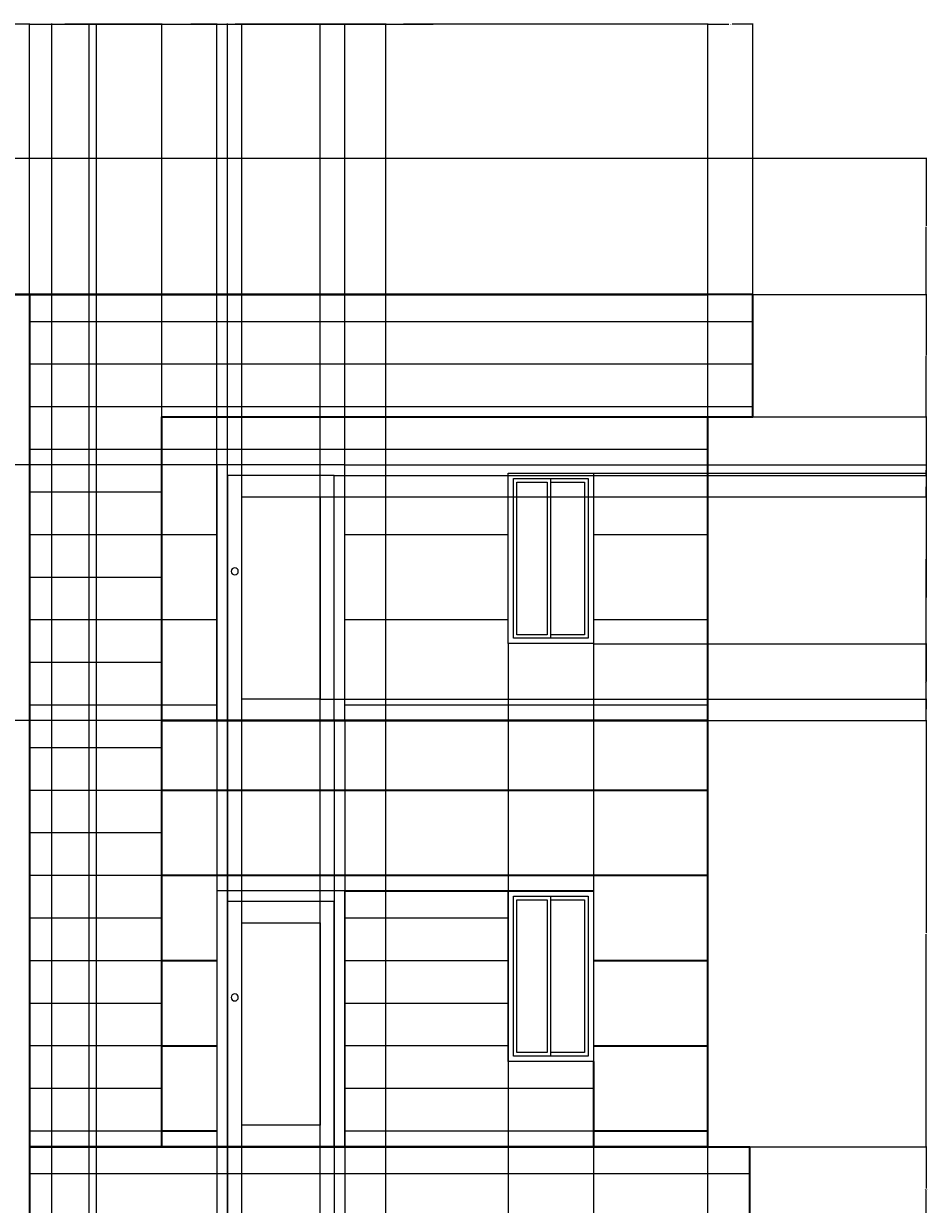
# Model space of a CAD drawing. Units: inches. Extents: x 10 to 404, y -77 to 696.
# Tile 5 of 5: x 149 to 404, y 363 to 696. Entities that reach past the tile are written whole.
import ezdxf

# ---------------------------------------------------------------- set-up
doc = ezdxf.new("R2010")
doc.units = ezdxf.units.IN
doc.header["$MEASUREMENT"] = 0
for name, color, linetype, lineweight in [('A-ANNO-DIMS', 2, 'Continuous', 18), ('A-DOOR', 4, 'Continuous', 25), ('A-ELEV', 7, 'Continuous', 35), ('A-ELEV-PATT', 8, 'Continuous', 13), ('A-GLAZ', 4, 'Continuous', 25)]:
    doc.layers.add(name, color=color, linetype=linetype, lineweight=lineweight)
doc.styles.get("Standard").update_dxf_attribs({"font": 'arial.ttf'})
doc.dimstyles.get("Standard").update_dxf_attribs({"dimtxt": 0.18, "dimasz": 0.18, "dimexe": 0.18, "dimexo": 0.0625, "dimgap": 0.09, "dimtad": 0, "dimtih": 1, "dimtoh": 1, "dimdec": 4, "dimzin": 0, "dimdsep": 46, "dimtxsty": 'Standard', "dimcen": 0.09, "dimadec": 0, "dimazin": 0, "dimtfac": 1, "dimtdec": 4, "dimtofl": 0, "dimtmove": 0, "dimatfit": 3, "dimfxl": 1, "dimtolj": 1, "dimtzin": 0, "dimarcsym": 0})

# ---------------------------------------------------------------- blocks, each defined once
blk = doc.blocks.new('*U5')
for p, q in [((1.5, 1.5), (1.5, 46.5)), ((1.5, 46.5), (12, 46.5)), ((12, 1.5), (12, 46.5)), ((12, 46.5), (22.5, 46.5)), ((22.5, 46.5), (22.5, 1.5)), ((12, 1.5), (1.5, 1.5)), ((22.5, 1.5), (12, 1.5))]:
    blk.add_line(p, q)
blk.add_lwpolyline([(0, 0), (0, 48), (24, 48), (24, 0)], close=True)
for points in [[(11, 45.5), (11, 2.5), (2.5, 2.5), (2.5, 45.5), (11, 45.5)], [(12, 45.5), (21.5, 45.5), (21.5, 2.5), (12, 2.5)]]:
    blk.add_lwpolyline(points)
blk = doc.blocks.new('*U4')
blk.add_lwpolyline([(3.12, 0.01), (0.12, 0.01), (0.12, 72.01), (36.12, 72.01), (36.12, 0.01), (33.12, 0.01)])
for points in [[(33.12, 68.99), (33.12, 0.01), (3.12, 0.01), (3.12, 68.99)], [(29.12, 6.01), (29.12, 62.99), (7.12, 62.99), (7.12, 6.01)]]:
    blk.add_lwpolyline(points, close=True)
blk.add_circle((31.12, 42.01), 1)
blk = doc.blocks.new('*D10')
at = {"layer": 'A-ANNO-DIMS', "color": 0, "lineweight": -2, "transparency": 16777216}
for p, q in [((65.94, 657.96), (9.76, 657.96)), ((9.94, 657.78), (9.94, 315.77)), ((9.94, -26.6), (9.94, 315.41)), ((176.46, -26.78), (9.76, -26.78))]:
    blk.add_line(p, q, dxfattribs=at)
at = {"layer": 'A-ANNO-DIMS', "color": 0, "transparency": 16777216}
for points in [[(9.91, 657.78), (9.97, 657.78), (9.94, 657.96)], [(9.91, -26.6), (9.97, -26.6), (9.94, -26.78)]]:
    blk.add_solid(points, dxfattribs=at)
at = {"layer": 'Defpoints', "color": 0, "transparency": 16777216}
for p in [(9.94, 657.96), (66.01, 657.96), (176.53, -26.78)]:
    blk.add_point(p, dxfattribs=at)
at = {"layer": 'A-ANNO-DIMS', "color": 0, "transparency": 16777216, "insert": (9.94, 315.59), "char_height": 0.18, "attachment_point": 5}
blk.add_mtext('\\A1;684.7', dxfattribs=at)
blk = doc.blocks.new('*D18')
at = {"layer": 'A-ANNO-DIMS', "color": 0, "lineweight": -2, "transparency": 16777216}
for p, q in [((78.1, 619.62), (78.1, 695.87)), ((78.28, 695.69), (114.12, 695.69)), ((150.75, 695.69), (114.91, 695.69)), ((150.93, 619.62), (150.93, 695.87))]:
    blk.add_line(p, q, dxfattribs=at)
at = {"layer": 'A-ANNO-DIMS', "color": 0, "transparency": 16777216}
for points in [[(78.28, 695.72), (78.28, 695.66), (78.1, 695.69)], [(150.75, 695.72), (150.75, 695.66), (150.93, 695.69)]]:
    blk.add_solid(points, dxfattribs=at)
at = {"layer": 'Defpoints', "color": 0, "transparency": 16777216}
for p in [(150.93, 695.69), (78.1, 619.55), (150.93, 619.55)]:
    blk.add_point(p, dxfattribs=at)
at = {"layer": 'A-ANNO-DIMS', "color": 0, "transparency": 16777216, "insert": (114.52, 695.69), "char_height": 0.18, "attachment_point": 5}
blk.add_mtext('\\A1;72.83', dxfattribs=at)
blk = doc.blocks.new('*D19')
at = {"layer": 'A-ANNO-DIMS', "color": 0, "lineweight": -2, "transparency": 16777216}
for p, q in [((150.93, 619.62), (150.93, 695.87)), ((151.11, 695.69), (169.13, 695.69)), ((187.94, 695.69), (169.92, 695.69)), ((188.12, 585.2), (188.12, 695.87))]:
    blk.add_line(p, q, dxfattribs=at)
at = {"layer": 'A-ANNO-DIMS', "color": 0, "transparency": 16777216}
for points in [[(151.11, 695.72), (151.11, 695.66), (150.93, 695.69)], [(187.94, 695.72), (187.94, 695.66), (188.12, 695.69)]]:
    blk.add_solid(points, dxfattribs=at)
at = {"layer": 'Defpoints', "color": 0, "transparency": 16777216}
for p in [(188.12, 695.69), (150.93, 619.55), (188.12, 585.13)]:
    blk.add_point(p, dxfattribs=at)
at = {"layer": 'A-ANNO-DIMS', "color": 0, "transparency": 16777216, "insert": (169.53, 695.69), "char_height": 0.18, "attachment_point": 5}
blk.add_mtext('\\A1;37.18', dxfattribs=at)
blk = doc.blocks.new('*D20')
at = {"layer": 'A-ANNO-DIMS', "color": 0, "lineweight": -2, "transparency": 16777216}
for p, q in [((188.12, 585.2), (188.12, 695.87)), ((188.3, 695.69), (264.54, 695.69)), ((341.69, 695.69), (265.45, 695.69)), ((341.87, 585.2), (341.87, 695.87))]:
    blk.add_line(p, q, dxfattribs=at)
at = {"layer": 'A-ANNO-DIMS', "color": 0, "transparency": 16777216}
for points in [[(188.3, 695.72), (188.3, 695.66), (188.12, 695.69)], [(341.69, 695.72), (341.69, 695.66), (341.87, 695.69)]]:
    blk.add_solid(points, dxfattribs=at)
at = {"layer": 'Defpoints', "color": 0, "transparency": 16777216}
for p in [(341.87, 695.69), (188.12, 585.13), (341.87, 585.13)]:
    blk.add_point(p, dxfattribs=at)
at = {"layer": 'A-ANNO-DIMS', "color": 0, "transparency": 16777216, "insert": (264.99, 695.69), "char_height": 0.18, "attachment_point": 5}
blk.add_mtext('\\A1;153.75', dxfattribs=at)
blk = doc.blocks.new('*D21')
at = {"layer": 'A-ANNO-DIMS', "color": 0, "lineweight": -2, "transparency": 16777216}
for p, q in [((341.87, 585.2), (341.87, 695.87)), ((342.05, 695.69), (347.76, 695.69)), ((354.38, 695.69), (348.67, 695.69)), ((354.56, 619.62), (354.56, 695.87))]:
    blk.add_line(p, q, dxfattribs=at)
at = {"layer": 'A-ANNO-DIMS', "color": 0, "transparency": 16777216}
for points in [[(342.05, 695.72), (342.05, 695.66), (341.87, 695.69)], [(354.38, 695.72), (354.38, 695.66), (354.56, 695.69)]]:
    blk.add_solid(points, dxfattribs=at)
at = {"layer": 'Defpoints', "color": 0, "transparency": 16777216}
for p in [(354.56, 695.69), (354.56, 619.55), (341.87, 585.13)]:
    blk.add_point(p, dxfattribs=at)
at = {"layer": 'A-ANNO-DIMS', "color": 0, "transparency": 16777216, "insert": (348.21, 695.69), "char_height": 0.18, "attachment_point": 5}
blk.add_mtext('\\A1;12.696', dxfattribs=at)
blk = doc.blocks.new('*D22')
at = {"layer": 'A-ANNO-DIMS', "color": 0, "lineweight": -2, "transparency": 16777216}
for p, q in [((188.12, 499.62), (188.12, 695.87)), ((188.3, 695.69), (195.51, 695.69)), ((203.49, 695.69), (196.28, 695.69)), ((203.67, 499.67), (203.67, 695.87))]:
    blk.add_line(p, q, dxfattribs=at)
at = {"layer": 'A-ANNO-DIMS', "color": 0, "transparency": 16777216}
for points in [[(188.3, 695.72), (188.3, 695.66), (188.12, 695.69)], [(203.49, 695.72), (203.49, 695.66), (203.67, 695.69)]]:
    blk.add_solid(points, dxfattribs=at)
at = {"layer": 'Defpoints', "color": 0, "transparency": 16777216}
for p in [(203.67, 695.69), (188.12, 499.55), (203.67, 499.6)]:
    blk.add_point(p, dxfattribs=at)
at = {"layer": 'A-ANNO-DIMS', "color": 0, "transparency": 16777216, "insert": (195.89, 695.69), "char_height": 0.18, "attachment_point": 5}
blk.add_mtext('\\A1;15.55', dxfattribs=at)
blk = doc.blocks.new('*D31')
at = {"layer": 'A-ANNO-DIMS', "color": 0, "lineweight": -2, "transparency": 16777216}
for p, q in [((353.65, 379.55), (403.47, 379.55)), ((403.29, 379.37), (403.29, 367.75)), ((403.29, 355.76), (403.29, 367.38)), ((353.65, 355.58), (403.47, 355.58))]:
    blk.add_line(p, q, dxfattribs=at)
at = {"layer": 'A-ANNO-DIMS', "color": 0, "transparency": 16777216}
for points in [[(403.26, 379.37), (403.32, 379.37), (403.29, 379.55)], [(403.26, 355.76), (403.32, 355.76), (403.29, 355.58)]]:
    blk.add_solid(points, dxfattribs=at)
at = {"layer": 'Defpoints', "color": 0, "transparency": 16777216}
for p in [(353.59, 379.55), (403.29, 379.55), (353.59, 355.58)]:
    blk.add_point(p, dxfattribs=at)
at = {"layer": 'A-ANNO-DIMS', "color": 0, "transparency": 16777216, "insert": (403.29, 367.57), "char_height": 0.18, "attachment_point": 5}
blk.add_mtext('\\A1;23.975', dxfattribs=at)
blk = doc.blocks.new('*D32')
at = {"layer": 'A-ANNO-DIMS', "color": 0, "lineweight": -2, "transparency": 16777216}
for p, q in [((341.93, 499.55), (403.47, 499.55)), ((403.29, 499.37), (403.29, 439.74)), ((403.29, 379.73), (403.29, 439.37)), ((341.93, 379.55), (403.47, 379.55))]:
    blk.add_line(p, q, dxfattribs=at)
at = {"layer": 'A-ANNO-DIMS', "color": 0, "transparency": 16777216}
for points in [[(403.26, 499.37), (403.32, 499.37), (403.29, 499.55)], [(403.26, 379.73), (403.32, 379.73), (403.29, 379.55)]]:
    blk.add_solid(points, dxfattribs=at)
at = {"layer": 'Defpoints', "color": 0, "transparency": 16777216}
for p in [(341.87, 499.55), (403.29, 499.55), (341.87, 379.55)]:
    blk.add_point(p, dxfattribs=at)
at = {"layer": 'A-ANNO-DIMS', "color": 0, "transparency": 16777216, "insert": (403.29, 439.55), "char_height": 0.18, "attachment_point": 5}
blk.add_mtext('\\A1;120', dxfattribs=at)
blk = doc.blocks.new('*D33')
at = {"layer": 'A-ANNO-DIMS', "color": 0, "lineweight": -2, "transparency": 16777216}
for p, q in [((354.63, 585.13), (403.47, 585.13)), ((403.29, 584.95), (403.29, 542.53)), ((403.29, 499.73), (403.29, 542.16)), ((341.93, 499.55), (403.47, 499.55))]:
    blk.add_line(p, q, dxfattribs=at)
at = {"layer": 'A-ANNO-DIMS', "color": 0, "transparency": 16777216}
for points in [[(403.26, 584.95), (403.32, 584.95), (403.29, 585.13)], [(403.26, 499.73), (403.32, 499.73), (403.29, 499.55)]]:
    blk.add_solid(points, dxfattribs=at)
at = {"layer": 'Defpoints', "color": 0, "transparency": 16777216}
for p in [(354.56, 585.13), (403.29, 585.13), (341.87, 499.55)]:
    blk.add_point(p, dxfattribs=at)
at = {"layer": 'A-ANNO-DIMS', "color": 0, "transparency": 16777216, "insert": (403.29, 542.34), "char_height": 0.18, "attachment_point": 5}
blk.add_mtext('\\A1;85.58', dxfattribs=at)
blk = doc.blocks.new('*D34')
at = {"layer": 'A-ANNO-DIMS', "color": 0, "lineweight": -2, "transparency": 16777216}
for p, q in [((354.63, 619.55), (403.47, 619.55)), ((403.29, 619.37), (403.29, 602.53)), ((403.29, 585.31), (403.29, 602.16)), ((354.63, 585.13), (403.47, 585.13))]:
    blk.add_line(p, q, dxfattribs=at)
at = {"layer": 'A-ANNO-DIMS', "color": 0, "transparency": 16777216}
for points in [[(403.26, 619.37), (403.32, 619.37), (403.29, 619.55)], [(403.26, 585.31), (403.32, 585.31), (403.29, 585.13)]]:
    blk.add_solid(points, dxfattribs=at)
at = {"layer": 'Defpoints', "color": 0, "transparency": 16777216}
for p in [(354.56, 619.55), (403.29, 619.55), (354.56, 585.13)]:
    blk.add_point(p, dxfattribs=at)
at = {"layer": 'A-ANNO-DIMS', "color": 0, "transparency": 16777216, "insert": (403.29, 602.34), "char_height": 0.18, "attachment_point": 5}
blk.add_mtext('\\A1;34.42', dxfattribs=at)
blk = doc.blocks.new('*D35')
at = {"layer": 'A-ANNO-DIMS', "color": 0, "lineweight": -2, "transparency": 16777216}
for p, q in [((66.07, 657.96), (403.47, 657.96)), ((403.29, 657.78), (403.29, 638.94)), ((403.29, 619.73), (403.29, 638.58)), ((354.63, 619.55), (403.47, 619.55))]:
    blk.add_line(p, q, dxfattribs=at)
at = {"layer": 'A-ANNO-DIMS', "color": 0, "transparency": 16777216}
for points in [[(403.26, 657.78), (403.32, 657.78), (403.29, 657.96)], [(403.26, 619.73), (403.32, 619.73), (403.29, 619.55)]]:
    blk.add_solid(points, dxfattribs=at)
at = {"layer": 'Defpoints', "color": 0, "transparency": 16777216}
for p in [(66.01, 657.96), (403.29, 657.96), (354.56, 619.55)]:
    blk.add_point(p, dxfattribs=at)
at = {"layer": 'A-ANNO-DIMS', "color": 0, "transparency": 16777216, "insert": (403.29, 638.76), "char_height": 0.18, "attachment_point": 5}
blk.add_mtext('\\A1;38.41', dxfattribs=at)
blk = doc.blocks.new('*D40')
at = {"layer": 'A-ANNO-DIMS', "color": 0, "lineweight": -2, "transparency": 16777216}
for p, q in [((150.93, 259.62), (150.93, 695.87)), ((151.11, 695.69), (159.89, 695.69)), ((169.58, 695.69), (160.8, 695.69)), ((169.76, 289.65), (169.76, 695.87))]:
    blk.add_line(p, q, dxfattribs=at)
at = {"layer": 'A-ANNO-DIMS', "color": 0, "transparency": 16777216}
for points in [[(151.11, 695.72), (151.11, 695.66), (150.93, 695.69)], [(169.58, 695.72), (169.58, 695.66), (169.76, 695.69)]]:
    blk.add_solid(points, dxfattribs=at)
at = {"layer": 'Defpoints', "color": 0, "transparency": 16777216}
for p in [(169.76, 695.69), (169.76, 289.59), (150.93, 259.55)]:
    blk.add_point(p, dxfattribs=at)
at = {"layer": 'A-ANNO-DIMS', "color": 0, "transparency": 16777216, "insert": (160.35, 695.69), "char_height": 0.18, "attachment_point": 5}
blk.add_mtext('\\A1;18.827', dxfattribs=at)
blk = doc.blocks.new('*D41')
at = {"layer": 'A-ANNO-DIMS', "color": 0, "lineweight": -2, "transparency": 16777216}
for p, q in [((169.76, 289.65), (169.76, 695.87)), ((169.94, 695.69), (255.45, 695.69)), ((341.69, 695.69), (256.18, 695.69)), ((341.87, 289.65), (341.87, 695.87))]:
    blk.add_line(p, q, dxfattribs=at)
at = {"layer": 'A-ANNO-DIMS', "color": 0, "transparency": 16777216}
for points in [[(169.94, 695.72), (169.94, 695.66), (169.76, 695.69)], [(341.69, 695.72), (341.69, 695.66), (341.87, 695.69)]]:
    blk.add_solid(points, dxfattribs=at)
at = {"layer": 'Defpoints', "color": 0, "transparency": 16777216}
for p in [(341.87, 695.69), (169.76, 289.59), (341.87, 289.59)]:
    blk.add_point(p, dxfattribs=at)
at = {"layer": 'A-ANNO-DIMS', "color": 0, "transparency": 16777216, "insert": (255.81, 695.69), "char_height": 0.18, "attachment_point": 5}
blk.add_mtext('\\A1;172.1', dxfattribs=at)
blk = doc.blocks.new('*D46')
at = {"layer": 'A-ANNO-DIMS', "color": 0, "lineweight": -2, "transparency": 16777216}
for p, q in [((309.68, 521.23), (403.47, 521.23)), ((403.29, 521.05), (403.29, 510.6)), ((403.29, 499.78), (403.29, 510.24)), ((239.73, 499.6), (403.47, 499.6))]:
    blk.add_line(p, q, dxfattribs=at)
at = {"layer": 'A-ANNO-DIMS', "color": 0, "transparency": 16777216}
for points in [[(403.26, 521.05), (403.32, 521.05), (403.29, 521.23)], [(403.26, 499.78), (403.32, 499.78), (403.29, 499.6)]]:
    blk.add_solid(points, dxfattribs=at)
at = {"layer": 'Defpoints', "color": 0, "transparency": 16777216}
for p in [(309.62, 521.23), (239.67, 499.6), (403.29, 499.6)]:
    blk.add_point(p, dxfattribs=at)
at = {"layer": 'A-ANNO-DIMS', "color": 0, "transparency": 16777216, "insert": (403.29, 510.42), "char_height": 0.18, "attachment_point": 5}
blk.add_mtext('\\A1;21.63', dxfattribs=at)
blk = doc.blocks.new('*D47')
at = {"layer": 'A-ANNO-DIMS', "color": 0, "lineweight": -2, "transparency": 16777216}
for p, q in [((309.68, 569.23), (403.47, 569.23)), ((403.29, 569.05), (403.29, 545.42)), ((403.29, 521.41), (403.29, 545.05)), ((309.68, 521.23), (403.47, 521.23))]:
    blk.add_line(p, q, dxfattribs=at)
at = {"layer": 'A-ANNO-DIMS', "color": 0, "transparency": 16777216}
for points in [[(403.26, 569.05), (403.32, 569.05), (403.29, 569.23)], [(403.26, 521.41), (403.32, 521.41), (403.29, 521.23)]]:
    blk.add_solid(points, dxfattribs=at)
at = {"layer": 'Defpoints', "color": 0, "transparency": 16777216}
for p in [(309.62, 569.23), (403.29, 569.23), (309.62, 521.23)]:
    blk.add_point(p, dxfattribs=at)
at = {"layer": 'A-ANNO-DIMS', "color": 0, "transparency": 16777216, "insert": (403.29, 545.23), "char_height": 0.18, "attachment_point": 5}
blk.add_mtext('\\A1;48', dxfattribs=at)
blk = doc.blocks.new('*D48')
at = {"layer": 'A-ANNO-DIMS', "color": 0, "lineweight": -2, "transparency": 16777216}
for p, q in [((285.62, 521.17), (285.62, -64.31)), ((239.67, 499.54), (239.67, -64.31)), ((239.85, -64.13), (262.25, -64.13)), ((285.44, -64.13), (263.04, -64.13))]:
    blk.add_line(p, q, dxfattribs=at)
at = {"layer": 'A-ANNO-DIMS', "color": 0, "transparency": 16777216}
for points in [[(239.85, -64.1), (239.85, -64.16), (239.67, -64.13)], [(285.44, -64.1), (285.44, -64.16), (285.62, -64.13)]]:
    blk.add_solid(points, dxfattribs=at)
at = {"layer": 'Defpoints', "color": 0, "transparency": 16777216}
for p in [(285.62, 521.23), (239.67, 499.6), (285.62, -64.13)]:
    blk.add_point(p, dxfattribs=at)
at = {"layer": 'A-ANNO-DIMS', "color": 0, "transparency": 16777216, "insert": (262.64, -64.13), "char_height": 0.18, "attachment_point": 5}
blk.add_mtext('\\A1;45.95', dxfattribs=at)
blk = doc.blocks.new('*D49')
at = {"layer": 'A-ANNO-DIMS', "color": 0, "lineweight": -2, "transparency": 16777216}
for p, q in [((285.62, 521.17), (285.62, -64.31)), ((309.62, 521.17), (309.62, -64.31)), ((285.8, -64.13), (297.4, -64.13)), ((309.44, -64.13), (297.84, -64.13))]:
    blk.add_line(p, q, dxfattribs=at)
at = {"layer": 'A-ANNO-DIMS', "color": 0, "transparency": 16777216}
for points in [[(285.8, -64.1), (285.8, -64.16), (285.62, -64.13)], [(309.44, -64.1), (309.44, -64.16), (309.62, -64.13)]]:
    blk.add_solid(points, dxfattribs=at)
at = {"layer": 'Defpoints', "color": 0, "transparency": 16777216}
for p in [(285.62, 521.23), (309.62, 521.23), (309.62, -64.13)]:
    blk.add_point(p, dxfattribs=at)
at = {"layer": 'A-ANNO-DIMS', "color": 0, "transparency": 16777216, "insert": (297.62, -64.13), "char_height": 0.18, "attachment_point": 5}
blk.add_mtext('\\A1;24', dxfattribs=at)
blk = doc.blocks.new('*D50')
at = {"layer": 'A-ANNO-DIMS', "color": 0, "lineweight": -2, "transparency": 16777216}
for p, q in [((157.2, 100.31), (157.2, 695.87)), ((157.38, 695.69), (161.98, 695.69)), ((167.49, 695.69), (162.89, 695.69)), ((167.67, 91.62), (167.67, 695.87))]:
    blk.add_line(p, q, dxfattribs=at)
at = {"layer": 'A-ANNO-DIMS', "color": 0, "transparency": 16777216}
for points in [[(157.38, 695.72), (157.38, 695.66), (157.2, 695.69)], [(167.49, 695.72), (167.49, 695.66), (167.67, 695.69)]]:
    blk.add_solid(points, dxfattribs=at)
at = {"layer": 'Defpoints', "color": 0, "transparency": 16777216}
for p in [(167.67, 695.69), (157.2, 100.24), (167.67, 91.55)]:
    blk.add_point(p, dxfattribs=at)
at = {"layer": 'A-ANNO-DIMS', "color": 0, "transparency": 16777216, "insert": (162.43, 695.69), "char_height": 0.18, "attachment_point": 5}
blk.add_mtext('\\A1;10.469', dxfattribs=at)
blk = doc.blocks.new('*D51')
at = {"layer": 'A-ANNO-DIMS', "color": 0, "lineweight": -2, "transparency": 16777216}
for p, q in [((167.67, 91.62), (167.67, 695.87)), ((167.85, 695.69), (209.06, 695.69)), ((251.06, 695.69), (209.85, 695.69)), ((251.24, 100.31), (251.24, 695.87))]:
    blk.add_line(p, q, dxfattribs=at)
at = {"layer": 'A-ANNO-DIMS', "color": 0, "transparency": 16777216}
for points in [[(167.85, 695.72), (167.85, 695.66), (167.67, 695.69)], [(251.06, 695.72), (251.06, 695.66), (251.24, 695.69)]]:
    blk.add_solid(points, dxfattribs=at)
at = {"layer": 'Defpoints', "color": 0, "transparency": 16777216}
for p in [(251.24, 695.69), (251.24, 100.24), (167.67, 91.55)]:
    blk.add_point(p, dxfattribs=at)
at = {"layer": 'A-ANNO-DIMS', "color": 0, "transparency": 16777216, "insert": (209.45, 695.69), "char_height": 0.18, "attachment_point": 5}
blk.add_mtext('\\A1;83.57', dxfattribs=at)
blk = doc.blocks.new('*D61')
at = {"layer": 'A-ANNO-DIMS', "color": 0, "lineweight": -2, "transparency": 16777216}
for p, q in [((206.67, 19.62), (206.67, 695.87)), ((206.85, 695.69), (208.51, 695.69)), ((210.49, 695.69), (208.82, 695.69)), ((210.67, 25.62), (210.67, 695.87))]:
    blk.add_line(p, q, dxfattribs=at)
at = {"layer": 'A-ANNO-DIMS', "color": 0, "transparency": 16777216}
for points in [[(206.85, 695.72), (206.85, 695.66), (206.67, 695.69)], [(210.49, 695.72), (210.49, 695.66), (210.67, 695.69)]]:
    blk.add_solid(points, dxfattribs=at)
at = {"layer": 'Defpoints', "color": 0, "transparency": 16777216}
for p in [(210.67, 695.69), (210.67, 25.55), (206.67, 19.55)]:
    blk.add_point(p, dxfattribs=at)
at = {"layer": 'A-ANNO-DIMS', "color": 0, "transparency": 16777216, "insert": (208.67, 695.69), "char_height": 0.18, "attachment_point": 5}
blk.add_mtext('\\A1;4', dxfattribs=at)
blk = doc.blocks.new('*D62')
at = {"layer": 'A-ANNO-DIMS', "color": 0, "lineweight": -2, "transparency": 16777216}
for p, q in [((210.67, 25.62), (210.67, 695.87)), ((210.85, 695.69), (221.45, 695.69)), ((232.49, 695.69), (221.89, 695.69)), ((232.67, 25.62), (232.67, 695.87))]:
    blk.add_line(p, q, dxfattribs=at)
at = {"layer": 'A-ANNO-DIMS', "color": 0, "transparency": 16777216}
for points in [[(210.85, 695.72), (210.85, 695.66), (210.67, 695.69)], [(232.49, 695.72), (232.49, 695.66), (232.67, 695.69)]]:
    blk.add_solid(points, dxfattribs=at)
at = {"layer": 'Defpoints', "color": 0, "transparency": 16777216}
for p in [(232.67, 695.69), (210.67, 25.55), (232.67, 25.55)]:
    blk.add_point(p, dxfattribs=at)
at = {"layer": 'A-ANNO-DIMS', "color": 0, "transparency": 16777216, "insert": (221.67, 695.69), "char_height": 0.18, "attachment_point": 5}
blk.add_mtext('\\A1;22', dxfattribs=at)
blk = doc.blocks.new('*D65')
at = {"layer": 'A-ANNO-DIMS', "color": 0, "lineweight": -2, "transparency": 16777216}
for p, q in [((203.67, 571.67), (203.67, 695.87)), ((203.85, 695.69), (221.45, 695.69)), ((239.49, 695.69), (221.89, 695.69)), ((239.67, 571.67), (239.67, 695.87))]:
    blk.add_line(p, q, dxfattribs=at)
at = {"layer": 'A-ANNO-DIMS', "color": 0, "transparency": 16777216}
for points in [[(203.85, 695.72), (203.85, 695.66), (203.67, 695.69)], [(239.49, 695.72), (239.49, 695.66), (239.67, 695.69)]]:
    blk.add_solid(points, dxfattribs=at)
at = {"layer": 'Defpoints', "color": 0, "transparency": 16777216}
for p in [(239.67, 695.69), (203.67, 571.6), (239.67, 571.6)]:
    blk.add_point(p, dxfattribs=at)
at = {"layer": 'A-ANNO-DIMS', "color": 0, "transparency": 16777216, "insert": (221.67, 695.69), "char_height": 0.18, "attachment_point": 5}
blk.add_mtext('\\A1;36', dxfattribs=at)
blk = doc.blocks.new('*D66')
at = {"layer": 'A-ANNO-DIMS', "color": 0, "lineweight": -2, "transparency": 16777216}
for p, q in [((203.67, 499.54), (203.67, -64.31)), ((206.67, 499.54), (206.67, -64.31)), ((203.85, -64.13), (205.02, -64.13)), ((206.49, -64.13), (205.32, -64.13))]:
    blk.add_line(p, q, dxfattribs=at)
at = {"layer": 'A-ANNO-DIMS', "color": 0, "transparency": 16777216}
for points in [[(203.85, -64.1), (203.85, -64.16), (203.67, -64.13)], [(206.49, -64.1), (206.49, -64.16), (206.67, -64.13)]]:
    blk.add_solid(points, dxfattribs=at)
at = {"layer": 'Defpoints', "color": 0, "transparency": 16777216}
for p in [(203.67, 499.6), (206.67, 499.6), (206.67, -64.13)]:
    blk.add_point(p, dxfattribs=at)
at = {"layer": 'A-ANNO-DIMS', "color": 0, "transparency": 16777216, "insert": (205.17, -64.13), "char_height": 0.18, "attachment_point": 5}
blk.add_mtext('\\A1;3', dxfattribs=at)
blk = doc.blocks.new('*D67')
at = {"layer": 'A-ANNO-DIMS', "color": 0, "lineweight": -2, "transparency": 16777216}
for p, q in [((206.67, 499.54), (206.67, -64.31)), ((236.67, 499.54), (236.67, -64.31)), ((206.85, -64.13), (221.45, -64.13)), ((236.49, -64.13), (221.89, -64.13))]:
    blk.add_line(p, q, dxfattribs=at)
at = {"layer": 'A-ANNO-DIMS', "color": 0, "transparency": 16777216}
for points in [[(206.85, -64.1), (206.85, -64.16), (206.67, -64.13)], [(236.49, -64.1), (236.49, -64.16), (236.67, -64.13)]]:
    blk.add_solid(points, dxfattribs=at)
at = {"layer": 'Defpoints', "color": 0, "transparency": 16777216}
for p in [(206.67, 499.6), (236.67, 499.6), (236.67, -64.13)]:
    blk.add_point(p, dxfattribs=at)
at = {"layer": 'A-ANNO-DIMS', "color": 0, "transparency": 16777216, "insert": (221.67, -64.13), "char_height": 0.18, "attachment_point": 5}
blk.add_mtext('\\A1;30', dxfattribs=at)
blk = doc.blocks.new('*D68')
at = {"layer": 'A-ANNO-DIMS', "color": 0, "lineweight": -2, "transparency": 16777216}
for p, q in [((236.67, 499.54), (236.67, -64.31)), ((239.67, 499.54), (239.67, -64.31)), ((236.85, -64.13), (238.02, -64.13)), ((239.49, -64.13), (238.32, -64.13))]:
    blk.add_line(p, q, dxfattribs=at)
at = {"layer": 'A-ANNO-DIMS', "color": 0, "transparency": 16777216}
for points in [[(236.85, -64.1), (236.85, -64.16), (236.67, -64.13)], [(239.49, -64.1), (239.49, -64.16), (239.67, -64.13)]]:
    blk.add_solid(points, dxfattribs=at)
at = {"layer": 'Defpoints', "color": 0, "transparency": 16777216}
for p in [(236.67, 499.6), (239.67, 499.6), (239.67, -64.13)]:
    blk.add_point(p, dxfattribs=at)
at = {"layer": 'A-ANNO-DIMS', "color": 0, "transparency": 16777216, "insert": (238.17, -64.13), "char_height": 0.18, "attachment_point": 5}
blk.add_mtext('\\A1;3', dxfattribs=at)
blk = doc.blocks.new('*D69')
at = {"layer": 'A-ANNO-DIMS', "color": 0, "lineweight": -2, "transparency": 16777216}
for p, q in [((206.67, 499.67), (206.67, 695.87)), ((206.85, 695.69), (208.51, 695.69)), ((210.49, 695.69), (208.82, 695.69)), ((210.67, 505.67), (210.67, 695.87))]:
    blk.add_line(p, q, dxfattribs=at)
at = {"layer": 'A-ANNO-DIMS', "color": 0, "transparency": 16777216}
for points in [[(206.85, 695.72), (206.85, 695.66), (206.67, 695.69)], [(210.49, 695.72), (210.49, 695.66), (210.67, 695.69)]]:
    blk.add_solid(points, dxfattribs=at)
at = {"layer": 'Defpoints', "color": 0, "transparency": 16777216}
for p in [(210.67, 695.69), (210.67, 505.6), (206.67, 499.6)]:
    blk.add_point(p, dxfattribs=at)
at = {"layer": 'A-ANNO-DIMS', "color": 0, "transparency": 16777216, "insert": (208.67, 695.69), "char_height": 0.18, "attachment_point": 5}
blk.add_mtext('\\A1;4', dxfattribs=at)
blk = doc.blocks.new('*D70')
at = {"layer": 'A-ANNO-DIMS', "color": 0, "lineweight": -2, "transparency": 16777216}
for p, q in [((210.67, 505.67), (210.67, 695.87)), ((210.85, 695.69), (221.45, 695.69)), ((232.49, 695.69), (221.89, 695.69)), ((232.67, 505.67), (232.67, 695.87))]:
    blk.add_line(p, q, dxfattribs=at)
at = {"layer": 'A-ANNO-DIMS', "color": 0, "transparency": 16777216}
for points in [[(210.85, 695.72), (210.85, 695.66), (210.67, 695.69)], [(232.49, 695.72), (232.49, 695.66), (232.67, 695.69)]]:
    blk.add_solid(points, dxfattribs=at)
at = {"layer": 'Defpoints', "color": 0, "transparency": 16777216}
for p in [(232.67, 695.69), (210.67, 505.6), (232.67, 505.6)]:
    blk.add_point(p, dxfattribs=at)
at = {"layer": 'A-ANNO-DIMS', "color": 0, "transparency": 16777216, "insert": (221.67, 695.69), "char_height": 0.18, "attachment_point": 5}
blk.add_mtext('\\A1;22', dxfattribs=at)
blk = doc.blocks.new('*D71')
at = {"layer": 'A-ANNO-DIMS', "color": 0, "lineweight": -2, "transparency": 16777216}
for p, q in [((203.6, 571.6), (9.76, 571.6)), ((9.94, 571.42), (9.94, 535.78)), ((9.94, 499.78), (9.94, 535.42)), ((203.6, 499.6), (9.76, 499.6))]:
    blk.add_line(p, q, dxfattribs=at)
at = {"layer": 'A-ANNO-DIMS', "color": 0, "transparency": 16777216}
for points in [[(9.91, 571.42), (9.97, 571.42), (9.94, 571.6)], [(9.91, 499.78), (9.97, 499.78), (9.94, 499.6)]]:
    blk.add_solid(points, dxfattribs=at)
at = {"layer": 'Defpoints', "color": 0, "transparency": 16777216}
for p in [(9.94, 571.6), (203.67, 571.6), (203.67, 499.6)]:
    blk.add_point(p, dxfattribs=at)
at = {"layer": 'A-ANNO-DIMS', "color": 0, "transparency": 16777216, "insert": (9.94, 535.6), "char_height": 0.18, "attachment_point": 5}
blk.add_mtext('\\A1;72', dxfattribs=at)
blk = doc.blocks.new('*D72')
at = {"layer": 'A-ANNO-DIMS', "color": 0, "lineweight": -2, "transparency": 16777216}
for p, q in [((232.73, 505.6), (403.47, 505.6)), ((403.29, 505.42), (403.29, 502.79)), ((403.29, 499.78), (403.29, 502.42)), ((236.73, 499.6), (403.47, 499.6))]:
    blk.add_line(p, q, dxfattribs=at)
at = {"layer": 'A-ANNO-DIMS', "color": 0, "transparency": 16777216}
for points in [[(403.26, 505.42), (403.32, 505.42), (403.29, 505.6)], [(403.26, 499.78), (403.32, 499.78), (403.29, 499.6)]]:
    blk.add_solid(points, dxfattribs=at)
at = {"layer": 'Defpoints', "color": 0, "transparency": 16777216}
for p in [(232.67, 505.6), (403.29, 505.6), (236.67, 499.6)]:
    blk.add_point(p, dxfattribs=at)
at = {"layer": 'A-ANNO-DIMS', "color": 0, "transparency": 16777216, "insert": (403.29, 502.6), "char_height": 0.18, "attachment_point": 5}
blk.add_mtext('\\A1;6', dxfattribs=at)
blk = doc.blocks.new('*D73')
at = {"layer": 'A-ANNO-DIMS', "color": 0, "lineweight": -2, "transparency": 16777216}
for p, q in [((232.73, 562.58), (403.47, 562.58)), ((403.29, 562.4), (403.29, 534.27)), ((403.29, 505.78), (403.29, 533.91)), ((232.73, 505.6), (403.47, 505.6))]:
    blk.add_line(p, q, dxfattribs=at)
at = {"layer": 'A-ANNO-DIMS', "color": 0, "transparency": 16777216}
for points in [[(403.26, 562.4), (403.32, 562.4), (403.29, 562.58)], [(403.26, 505.78), (403.32, 505.78), (403.29, 505.6)]]:
    blk.add_solid(points, dxfattribs=at)
at = {"layer": 'Defpoints', "color": 0, "transparency": 16777216}
for p in [(232.67, 562.58), (403.29, 562.58), (232.67, 505.6)]:
    blk.add_point(p, dxfattribs=at)
at = {"layer": 'A-ANNO-DIMS', "color": 0, "transparency": 16777216, "insert": (403.29, 534.09), "char_height": 0.18, "attachment_point": 5}
blk.add_mtext('\\A1;56.98', dxfattribs=at)
blk = doc.blocks.new('*D74')
at = {"layer": 'A-ANNO-DIMS', "color": 0, "lineweight": -2, "transparency": 16777216}
for p, q in [((236.73, 568.58), (403.47, 568.58)), ((403.29, 568.4), (403.29, 565.76)), ((403.29, 562.76), (403.29, 565.4)), ((232.73, 562.58), (403.47, 562.58))]:
    blk.add_line(p, q, dxfattribs=at)
at = {"layer": 'A-ANNO-DIMS', "color": 0, "transparency": 16777216}
for points in [[(403.26, 568.4), (403.32, 568.4), (403.29, 568.58)], [(403.26, 562.76), (403.32, 562.76), (403.29, 562.58)]]:
    blk.add_solid(points, dxfattribs=at)
at = {"layer": 'Defpoints', "color": 0, "transparency": 16777216}
for p in [(236.67, 568.58), (403.29, 568.58), (232.67, 562.58)]:
    blk.add_point(p, dxfattribs=at)
at = {"layer": 'A-ANNO-DIMS', "color": 0, "transparency": 16777216, "insert": (403.29, 565.58), "char_height": 0.18, "attachment_point": 5}
blk.add_mtext('\\A1;6', dxfattribs=at)
blk = doc.blocks.new('*D75')
at = {"layer": 'A-ANNO-DIMS', "color": 0, "lineweight": -2, "transparency": 16777216}
for p, q in [((239.73, 571.6), (403.47, 571.6)), ((403.29, 571.42), (403.29, 570.28)), ((403.29, 568.76), (403.29, 569.91)), ((236.73, 568.58), (403.47, 568.58))]:
    blk.add_line(p, q, dxfattribs=at)
at = {"layer": 'A-ANNO-DIMS', "color": 0, "transparency": 16777216}
for points in [[(403.26, 571.42), (403.32, 571.42), (403.29, 571.6)], [(403.26, 568.76), (403.32, 568.76), (403.29, 568.58)]]:
    blk.add_solid(points, dxfattribs=at)
at = {"layer": 'Defpoints', "color": 0, "transparency": 16777216}
for p in [(239.67, 571.6), (403.29, 571.6), (236.67, 568.58)]:
    blk.add_point(p, dxfattribs=at)
at = {"layer": 'A-ANNO-DIMS', "color": 0, "transparency": 16777216, "insert": (403.29, 570.09), "char_height": 0.18, "attachment_point": 5}
blk.add_mtext('\\A1;3.023', dxfattribs=at)

msp = doc.modelspace()

# ---------------------------------------------------------------- hatches: boundary and pattern name
at = {"layer": 'A-ELEV-PATT'}
h = msp.add_hatch(dxfattribs=at)
h.set_pattern_fill('_USER', color=256, scale=12, pattern_type=0)
h.set_pattern_definition([(0, (0, 0), (0, 12), [])])
h.paths.add_polyline_path([(188.1159, 499.5535), (150.9344, 499.5535), (150.9344, 379.5535), (188.1159, 379.5535)])
h.paths.add_polyline_path([(188.1159, 585.1332), (354.5631, 585.1332), (354.5631, 619.5535), (341.8668, 619.5535), (150.9344, 619.5535), (150.9344, 499.5535), (188.1159, 499.5535)])
h.paths.add_polyline_path([(353.5898, 379.5535), (341.8668, 379.5535), (150.9344, 379.5535), (150.9344, 259.5535), (341.8668, 259.5535), (353.8668, 259.5535), (353.8668, 273.1993), (341.8668, 273.1993), (169.7618, 273.1993), (169.7618, 355.5535), (341.8668, 355.5535), (341.8668, 355.5783), (353.5898, 355.5783)])
h.paths.add_polyline_path([(285.6197, 451.5918), (239.6671, 451.5918), (239.6671, 379.5535), (309.6197, 379.5535), (309.6197, 403.5918), (285.6197, 403.5918)])
h.paths.add_polyline_path([(199.3943, 256.7444), (154.0619, 256.7444), (154.0619, 142.2479), (199.3943, 142.2479)])
h = msp.add_hatch(dxfattribs=at)
h.set_pattern_fill('_USER', color=256, scale=24, pattern_type=0)
h.set_pattern_definition([(0, (0, 0), (0, 24), [])])
h.paths.add_polyline_path([(341.8668, 139.5535), (150.9344, 139.5535), (150.9344, 19.5535), (167.6671, 19.5535), (167.6671, 91.5535), (157.1984, 91.5535), (157.1984, 100.244), (251.2392, 100.244), (251.2392, 91.5535), (239.6671, 91.5535), (239.6671, 19.5535), (341.8668, 19.5535)])
h.paths.add_polyline_path([(285.6197, 89.2337), (309.6197, 89.2337), (309.6197, 41.2337), (285.6197, 41.2337)], flags=16)
h.paths.add_polyline_path([(287.1197, 87.7337), (297.6197, 87.7337), (308.1197, 87.7337), (308.1197, 42.7337), (297.6197, 42.7337), (287.1197, 42.7337)], flags=0)
h.paths.add_polyline_path([(288.1197, 86.7337), (296.6197, 86.7337), (296.6197, 43.7337), (288.1197, 43.7337)], flags=0)
h.paths.add_polyline_path([(297.6197, 86.7337), (307.1197, 86.7337), (307.1197, 43.7337), (297.6197, 43.7337)], flags=0)
h.paths.add_polyline_path([(341.8668, 585.1332), (188.1159, 585.1332), (188.1159, 499.5535), (203.6671, 499.5535), (203.6671, 571.6046), (239.6671, 571.6046), (239.6671, 499.5535), (341.8668, 499.5535)])
h.paths.add_polyline_path([(285.6197, 521.2337), (285.6197, 569.2337), (309.6197, 569.2337), (309.6197, 521.2337)], flags=16)
h.paths.add_polyline_path([(287.1197, 522.7337), (287.1197, 567.7337), (297.6197, 567.7337), (308.1197, 567.7337), (308.1197, 522.7337), (297.6197, 522.7337)], flags=0)
h.paths.add_polyline_path([(288.1197, 523.7337), (288.1197, 566.7337), (296.6197, 566.7337), (296.6197, 523.7337)], flags=0)
h.paths.add_polyline_path([(297.6197, 566.7337), (307.1197, 566.7337), (307.1197, 523.7337), (297.6197, 523.7337)], flags=0)

# ---------------------------------------------------------------- linework, layer by layer
at = {"layer": 'A-ELEV'}
for p, q in [((341.8668, 619.5535), (78.1013, 619.5535)), ((78.1013, 619.5535), (341.8668, 619.5535)), ((150.9344, 19.5535), (150.9344, 619.5535)), ((354.5631, 619.5535), (341.8668, 619.5535)), ((354.5631, 585.1332), (354.5631, 619.5535)), ((188.1159, 379.5535), (188.1159, 585.1332)), ((188.1159, 585.1332), (354.5631, 585.1332)), ((341.8668, 499.5535), (341.8668, 585.1332)), ((341.8668, 499.5535), (188.1159, 499.5535)), ((188.1159, 499.5535), (341.8668, 499.5535)), ((341.8668, 379.5535), (341.8668, 499.5535)), ((188.1159, 480), (341.8668, 480)), ((188.1159, 456), (341.8668, 456)), ((239.6671, 451.5918), (309.6197, 451.5918)), ((188.1159, 432), (203.6671, 432)), ((309.6197, 432), (341.8668, 432)), ((188.1159, 408), (203.6671, 408)), ((309.6197, 408), (341.8668, 408)), ((309.6197, 403.5918), (309.6197, 379.5535)), ((188.1159, 384), (203.6671, 384)), ((309.6197, 384), (341.8668, 384)), ((341.8668, 379.5535), (150.9344, 379.5535)), ((150.9344, 379.5535), (341.8668, 379.5535))]:
    msp.add_line(p, q, dxfattribs=at)
msp.add_lwpolyline([(341.8668, 379.5535), (353.5898, 379.5535), (353.5898, 355.5783), (341.8668, 355.5783)], dxfattribs=at)

# ---------------------------------------------------------------- block references
at = {"layer": 'A-DOOR', "xscale": -1}
for p in [(239.7909, 499.5918), (239.7909, 379.5791)]:
    msp.add_blockref('*U4', p, dxfattribs=at)
at = {"layer": 'A-GLAZ'}
for p in [(285.6197, 521.2337), (285.6197, 403.5918)]:
    msp.add_blockref('*U5', p, dxfattribs=at)

# ---------------------------------------------------------------- dimensions: what is measured, and where the dimension line sits
at = {"layer": 'A-ANNO-DIMS'}
for base, p1, p2, override, picture, middle in [((150.9344, 695.6911), (78.1013, 619.5535), (150.9344, 619.5535), {"dimdec": 2, "dimlfac": 1, "dimrnd": 0, "dimzin": 0, "dimdsep": 46, "dimlunit": 2}, '*D18', (114.5179, 695.6911)), ((188.1159, 695.6911), (150.9344, 619.5535), (188.1159, 585.1332), {"dimdec": 2, "dimlfac": 1, "dimrnd": 0, "dimzin": 0, "dimdsep": 46, "dimlunit": 2}, '*D19', (169.5251, 695.6911)), ((169.7618, 695.6911), (150.9344, 259.5535), (169.7618, 289.5881), {"dimdec": 3, "dimlfac": 1, "dimrnd": 0, "dimzin": 0, "dimdsep": 46, "dimlunit": 2}, '*D40', (160.3481, 695.6911)), ((167.6671, 695.6911), (157.1984, 100.244), (167.6671, 91.5535), {"dimdec": 3, "dimlfac": 1, "dimrnd": 0, "dimzin": 0, "dimdsep": 46, "dimlunit": 2}, '*D50', (162.4328, 695.6911)), ((251.2392, 695.6911), (167.6671, 91.5535), (251.2392, 100.244), {"dimdec": 2, "dimlfac": 1, "dimrnd": 0, "dimzin": 0, "dimdsep": 46, "dimlunit": 2}, '*D51', (209.4531, 695.6911)), ((341.8668, 695.6911), (169.7618, 289.5881), (341.8668, 289.5881), {"dimdec": 1, "dimlfac": 1, "dimrnd": 0, "dimzin": 0, "dimdsep": 46, "dimlunit": 2}, '*D41', (255.8143, 695.6911)), ((341.8668, 695.6911), (188.1159, 585.1332), (341.8668, 585.1332), {"dimdec": 2, "dimlfac": 1, "dimrnd": 0, "dimzin": 0, "dimdsep": 46, "dimlunit": 2}, '*D20', (264.9913, 695.6911)), ((203.6671, 695.6911), (188.1159, 499.5535), (203.6671, 499.6046), {"dimdec": 2, "dimlfac": 1, "dimrnd": 0, "dimzin": 0, "dimdsep": 46, "dimlunit": 2}, '*D22', (195.8915, 695.6911)), ((239.6671, 695.6911), (203.6671, 571.6046), (239.6671, 571.6046), {"dimdec": 0, "dimlfac": 1, "dimrnd": 0, "dimzin": 0, "dimdsep": 46, "dimlunit": 2}, '*D65', (221.6671, 695.6911)), ((210.6671, 695.6911), (206.6671, 19.5535), (210.6671, 25.5535), {"dimdec": 0, "dimlfac": 1, "dimrnd": 0, "dimzin": 0, "dimdsep": 46, "dimlunit": 2}, '*D61', (208.6671, 695.6911)), ((210.6671, 695.6911), (206.6671, 499.6046), (210.6671, 505.6046), {"dimdec": 0, "dimlfac": 1, "dimrnd": 0, "dimzin": 0, "dimdsep": 46, "dimlunit": 2}, '*D69', (208.6671, 695.6911)), ((232.6671, 695.6911), (210.6671, 25.5535), (232.6671, 25.5535), {"dimdec": 0, "dimlfac": 1, "dimrnd": 0, "dimzin": 0, "dimdsep": 46, "dimlunit": 2}, '*D62', (221.6671, 695.6911)), ((232.6671, 695.6911), (210.6671, 505.6046), (232.6671, 505.6046), {"dimdec": 0, "dimlfac": 1, "dimrnd": 0, "dimzin": 0, "dimdsep": 46, "dimlunit": 2}, '*D70', (221.6671, 695.6911)), ((354.5631, 695.6911), (341.8668, 585.1332), (354.5631, 619.5535), {"dimdec": 3, "dimlfac": 1, "dimrnd": 0, "dimzin": 0, "dimdsep": 46, "dimlunit": 2}, '*D21', (348.2149, 695.6911)), ((285.6197, -64.1316), (239.6671, 499.6046), (285.6197, 521.2337), {"dimdec": 2, "dimlfac": 1, "dimrnd": 0, "dimzin": 0, "dimdsep": 46, "dimlunit": 2}, '*D48', (262.6434, -64.1316)), ((309.6197, -64.1316), (285.6197, 521.2337), (309.6197, 521.2337), {"dimdec": 0, "dimlfac": 1, "dimrnd": 0, "dimzin": 0, "dimdsep": 46, "dimlunit": 2}, '*D49', (297.6197, -64.1316)), ((206.6671, -64.1316), (203.6671, 499.6046), (206.6671, 499.6046), {"dimdec": 0, "dimlfac": 1, "dimrnd": 0, "dimzin": 0, "dimdsep": 46, "dimlunit": 2}, '*D66', (205.1671, -64.1316)), ((236.6671, -64.1316), (206.6671, 499.6046), (236.6671, 499.6046), {"dimdec": 0, "dimlfac": 1, "dimrnd": 0, "dimzin": 0, "dimdsep": 46, "dimlunit": 2}, '*D67', (221.6671, -64.1316)), ((239.6671, -64.1316), (236.6671, 499.6046), (239.6671, 499.6046), {"dimdec": 0, "dimlfac": 1, "dimrnd": 0, "dimzin": 0, "dimdsep": 46, "dimlunit": 2}, '*D68', (238.1671, -64.1316))]:
    dim = msp.add_linear_dim(base=base, p1=p1, p2=p2, dimstyle='Standard', override=override, dxfattribs=at)
    dim.commit()
    dim.dimension.update_dxf_attribs({"geometry": picture, "text_midpoint": middle})
for base, p1, p2, override, picture, middle in [((9.9405, 657.9612), (176.5266, -26.7816), (66.0062, 657.9612), {"dimdec": 1, "dimlfac": 1, "dimrnd": 0, "dimzin": 0, "dimdsep": 46, "dimlunit": 2}, '*D10', (9.9405, 315.5898)), ((403.2856, 657.9612), (354.5631, 619.5535), (66.0062, 657.9612), {"dimdec": 2, "dimlfac": 1, "dimrnd": 0, "dimzin": 0, "dimdsep": 46, "dimlunit": 2}, '*D35', (403.2856, 638.7574)), ((403.2856, 619.5535), (354.5631, 585.1332), (354.5631, 619.5535), {"dimdec": 2, "dimlfac": 1, "dimrnd": 0, "dimzin": 0, "dimdsep": 46, "dimlunit": 2}, '*D34', (403.2856, 602.3434)), ((403.2856, 585.1332), (341.8668, 499.5535), (354.5631, 585.1332), {"dimdec": 2, "dimlfac": 1, "dimrnd": 0, "dimzin": 0, "dimdsep": 46, "dimlunit": 2}, '*D33', (403.2856, 542.3434)), ((9.9405, 571.6046), (203.6671, 499.6046), (203.6671, 571.6046), {"dimdec": 0, "dimlfac": 1, "dimrnd": 0, "dimzin": 0, "dimdsep": 46, "dimlunit": 2}, '*D71', (9.9405, 535.6046)), ((403.2856, 571.6046), (236.6671, 568.5816), (239.6671, 571.6046), {"dimdec": 3, "dimlfac": 1, "dimrnd": 0, "dimzin": 0, "dimdsep": 46, "dimlunit": 2}, '*D75', (403.2856, 570.0931)), ((403.2856, 569.2337), (309.6197, 521.2337), (309.6197, 569.2337), {"dimdec": 0, "dimlfac": 1, "dimrnd": 0, "dimzin": 0, "dimdsep": 46, "dimlunit": 2}, '*D47', (403.2856, 545.2337)), ((403.2856, 568.5816), (232.6671, 562.5816), (236.6671, 568.5816), {"dimdec": 0, "dimlfac": 1, "dimrnd": 0, "dimzin": 0, "dimdsep": 46, "dimlunit": 2}, '*D74', (403.2856, 565.5816)), ((403.2856, 562.5816), (232.6671, 505.6046), (232.6671, 562.5816), {"dimdec": 2, "dimlfac": 1, "dimrnd": 0, "dimzin": 0, "dimdsep": 46, "dimlunit": 2}, '*D73', (403.2856, 534.0931)), ((403.2856, 499.6046), (309.6197, 521.2337), (239.6671, 499.6046), {"dimdec": 2, "dimlfac": 1, "dimrnd": 0, "dimzin": 0, "dimdsep": 46, "dimlunit": 2}, '*D46', (403.2856, 510.4191)), ((403.2856, 505.6046), (236.6671, 499.6046), (232.6671, 505.6046), {"dimdec": 0, "dimlfac": 1, "dimrnd": 0, "dimzin": 0, "dimdsep": 46, "dimlunit": 2}, '*D72', (403.2856, 502.6046)), ((403.2856, 499.5535), (341.8668, 379.5535), (341.8668, 499.5535), {"dimdec": 0, "dimlfac": 1, "dimrnd": 0, "dimzin": 0, "dimdsep": 46, "dimlunit": 2}, '*D32', (403.2856, 439.5535)), ((403.2856, 379.5535), (353.5898, 355.5783), (353.5898, 379.5535), {"dimdec": 3, "dimlfac": 1, "dimrnd": 0, "dimzin": 0, "dimdsep": 46, "dimlunit": 2}, '*D31', (403.2856, 367.5659))]:
    dim = msp.add_linear_dim(base=base, p1=p1, p2=p2, angle=90, dimstyle='Standard', override=override, dxfattribs=at)
    dim.commit()
    dim.dimension.update_dxf_attribs({"geometry": picture, "text_midpoint": middle})

doc.saveas('drawing.dxf')
